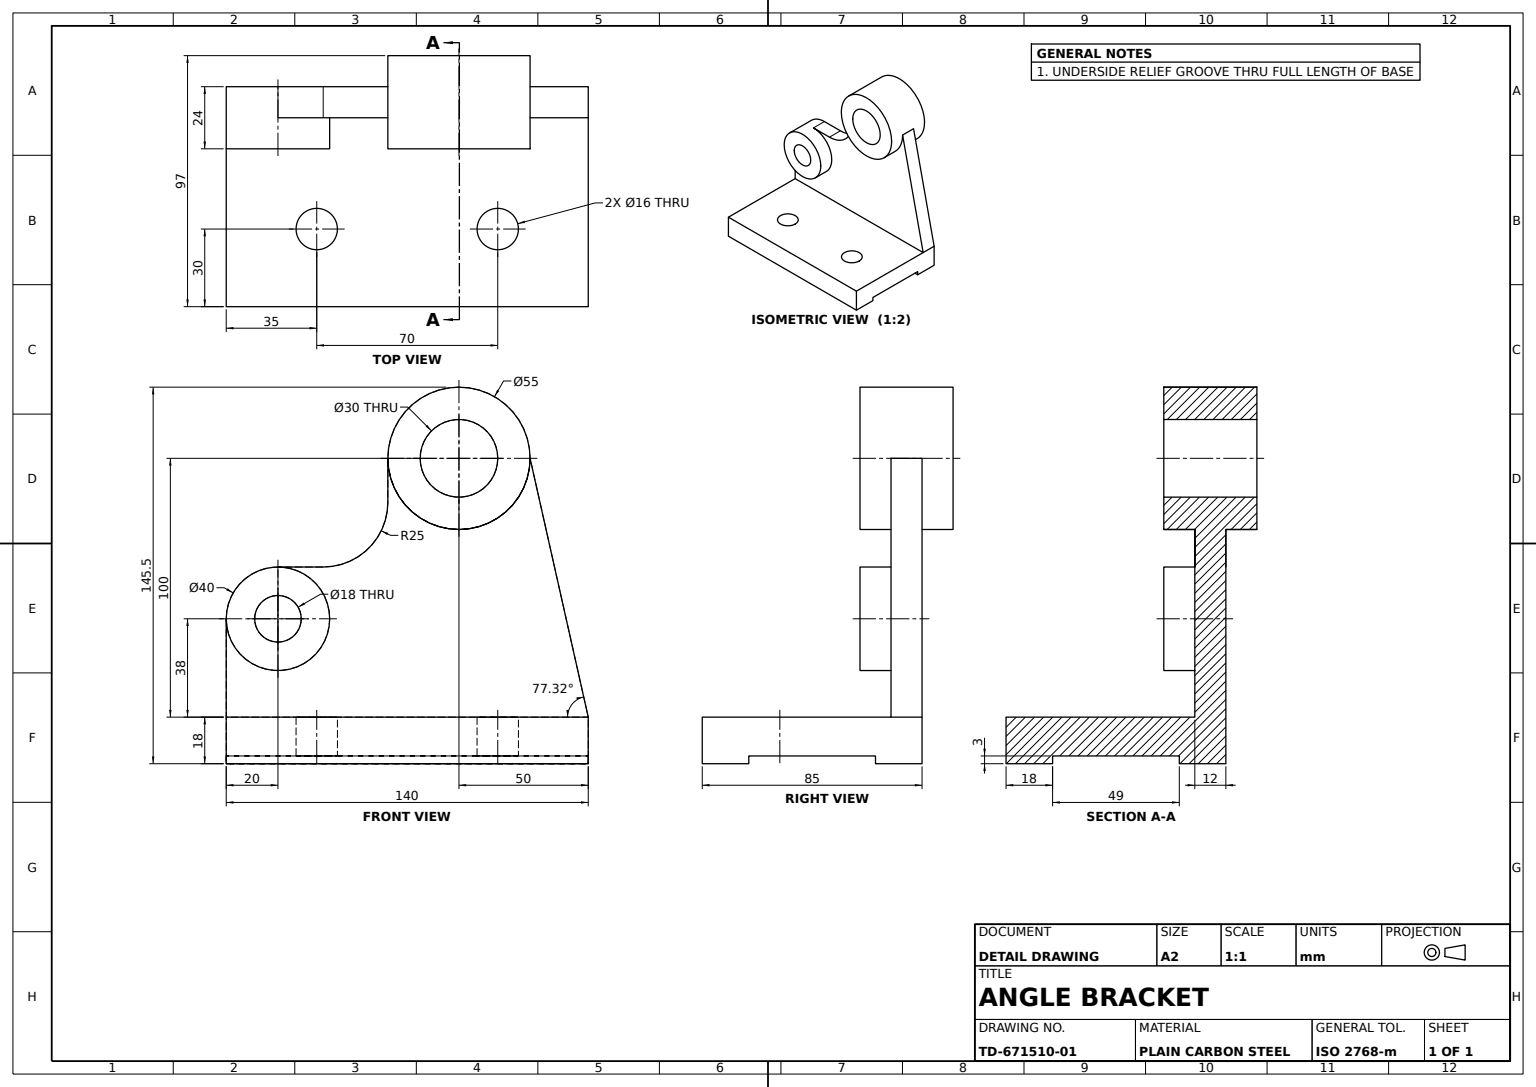
from build123d import *

# Parameters (mm, degrees)
BASE_PLATE_SKETCH_W              = 85
BASE_PLATE_SKETCH_H              = 140
BASE_PLATE_140X85X18_DEPTH       = 18
UNDERSIDE_RELIEF_GROOVE_SKETCH_W = 49
UNDERSIDE_RELIEF_GROOVE_SKETCH_H = 3
UNDERSIDE_RELIEF_GROOVE_DEPTH    = 150
ANGLED_SUPPORT_WEB_SKETCH_R      = 20
ANGLED_SUPPORT_WEB_SKETCH_R_2    = 9
ANGLED_SUPPORT_WEB_SKETCH_R_3    = 27.5
ANGLED_SUPPORT_WEB_SKETCH_R_4    = 15
ANGLED_SUPPORT_WEB_DEPTH         = 12
UPPER_BOSS_SKETCH_R              = 20
UPPER_BOSS_SKETCH_R_2            = 9
UPPER_BOSS_40_DEPTH              = 12
LOWER_START                      = 12
LOWER_BOSS_SKETCH_A_R            = 27.5
LOWER_BOSS_SKETCH_A_R_2          = 15
LOWER_BOSS_30_A_DEPTH            = 12
LOWER_BOSS_SKETCH_B_R            = 27.5
LOWER_BOSS_SKETCH_B_R_2          = 15
LOWER_BOSS_30_B_DEPTH            = 12
BASE_MOUNTING_HOLES_SKETCH_R     = 8
BASE_MOUNTING_HOLES_2X_16_DEPTH  = 20


with BuildPart() as part:
    # Base Plate Sketch → Base Plate 140x85x18 (new body)
    with BuildSketch(Plane(origin=(0, 0, 0), x_dir=(1, 0, 0), z_dir=(0, 1, 0))):
        Rectangle(BASE_PLATE_SKETCH_W, BASE_PLATE_SKETCH_H)
    extrude(amount=BASE_PLATE_140X85X18_DEPTH)

    # Underside Relief Groove Sketch → Underside Relief Groove (cut)
    with BuildSketch(Plane.XY.offset(70)):
        with Locations((0, 1.5)):
            Rectangle(UNDERSIDE_RELIEF_GROOVE_SKETCH_W, UNDERSIDE_RELIEF_GROOVE_SKETCH_H)
    extrude(amount=-UNDERSIDE_RELIEF_GROOVE_DEPTH, mode=Mode.SUBTRACT)

    # Angled Support Web Sketch → Angled Support Web (add)
    # profile 1 of 3: a face of its own
    with BuildSketch(Plane.ZY.offset(42.5)):
        with BuildLine():
            Line((-70, 18), (70, 18))
            Line((70, 18), (70, 56))
            ThreePointArc((70, 56), (35.857864376, 41.857864376), (50, 76))
            Line((50, 76), (32.5, 76))
            ThreePointArc((32.5, 76), (14.82233047, 83.32233047), (7.5, 101))
            Line((7.5, 101), (7.5, 118))
            ThreePointArc((7.5, 118), (-20, 90.5), (-47.5, 118))
            Line((-47.5, 118), (-70, 18))
        make_face()
    # profile 2 of 3: a face of its own
    with BuildSketch(Plane.ZY.offset(42.5)):
        with Locations((50, 56)):
            Circle(ANGLED_SUPPORT_WEB_SKETCH_R)
        with Locations((50, 56)):
            Circle(ANGLED_SUPPORT_WEB_SKETCH_R_2, mode=Mode.SUBTRACT)
    # profile 3 of 3: a face of its own
    with BuildSketch(Plane.ZY.offset(42.5)):
        with Locations((-20, 118)):
            Circle(ANGLED_SUPPORT_WEB_SKETCH_R_3)
        with Locations((-20, 118)):
            Circle(ANGLED_SUPPORT_WEB_SKETCH_R_4, mode=Mode.SUBTRACT)
    extrude(amount=-ANGLED_SUPPORT_WEB_DEPTH)

    # Upper Boss Sketch → Upper Boss Ø40 (add)
    with BuildSketch(Plane(origin=(-30.5, 0, 0), x_dir=(0, 0, -1), z_dir=(1, 0, 0))):
        with Locations(Location((-50, 56, 0), (0, 0, 180))):
            Circle(UPPER_BOSS_SKETCH_R)
        with Locations(Location((-50, 56, 0), (0, 0, 180))):
            Circle(UPPER_BOSS_SKETCH_R_2, mode=Mode.SUBTRACT)
    extrude(amount=UPPER_BOSS_40_DEPTH)

    # Lower Boss Sketch A → Lower Boss Ø30 A (add)
    with BuildSketch(Plane.ZY.offset(42.5).offset(LOWER_START)):
        with Locations((-20, 118)):
            Circle(LOWER_BOSS_SKETCH_A_R)
        with Locations((-20, 118)):
            Circle(LOWER_BOSS_SKETCH_A_R_2, mode=Mode.SUBTRACT)
    extrude(amount=-LOWER_BOSS_30_A_DEPTH)

    # Lower Boss Sketch B → Lower Boss Ø30 B (add)
    with BuildSketch(Plane(origin=(-30.5, 0, 0), x_dir=(0, 0, -1), z_dir=(1, 0, 0))):
        with Locations(Location((20, 118, 0), (0, 0, 180))):
            Circle(LOWER_BOSS_SKETCH_B_R)
        with Locations(Location((20, 118, 0), (0, 0, 180))):
            Circle(LOWER_BOSS_SKETCH_B_R_2, mode=Mode.SUBTRACT)
    extrude(amount=LOWER_BOSS_30_B_DEPTH)

    # Base Mounting Holes Sketch → Base Mounting Holes 2xØ16 (cut)
    with BuildSketch(Plane(origin=(0, 18, 0), x_dir=(1, 0, 0), z_dir=(0, 1, 0))):
        with Locations(Location((12.5, 35, 0), (0, 0, 270))):
            Circle(BASE_MOUNTING_HOLES_SKETCH_R)
        with Locations(Location((12.5, -35, 0), (0, 0, 270))):
            Circle(BASE_MOUNTING_HOLES_SKETCH_R)
    extrude(amount=-BASE_MOUNTING_HOLES_2X_16_DEPTH, mode=Mode.SUBTRACT)


solid = part.part
